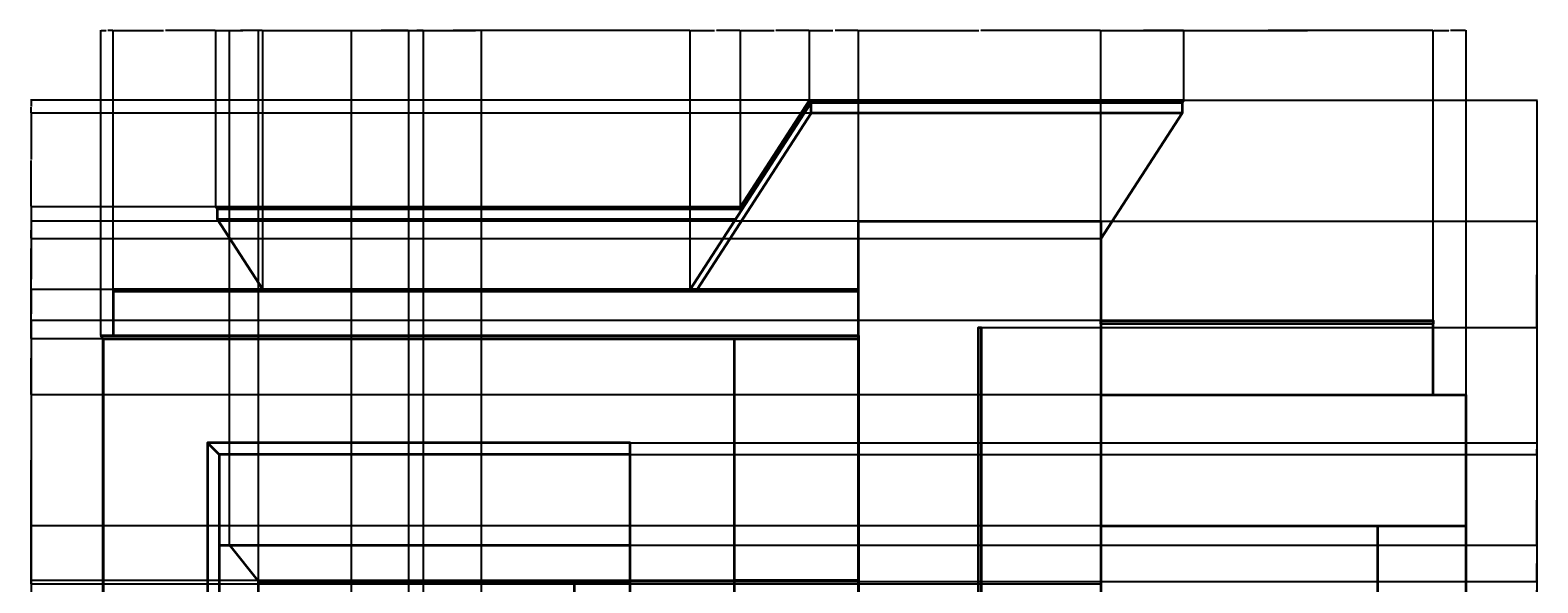
# Model space of a CAD drawing. Units: feet. Extents: x 4092 to 5585, y 725 to 1390.
# Tile 7 of 7: x 4921 to 5585, y 1146 to 1390. Entities that reach past the tile are written whole.
import ezdxf

# ---------------------------------------------------------------- set-up
doc = ezdxf.new("R2010")
doc.units = ezdxf.units.FT
doc.layers.add('A-ANNO-DIMS', color=2, linetype='Continuous', lineweight=18)
doc.layers.add('A-ELEV', color=7, linetype='Continuous', lineweight=35)
doc.styles.get("Standard").update_dxf_attribs({"font": 'arial.ttf'})
doc.dimstyles.get("Standard").update_dxf_attribs({"dimtxt": 0.18, "dimasz": 0.18, "dimexe": 0.18, "dimexo": 0.0625, "dimgap": 0.09, "dimtad": 0, "dimtih": 1, "dimtoh": 1, "dimdec": 1, "dimzin": 0, "dimdsep": 46, "dimlunit": 3, "dimtxsty": 'Standard', "dimcen": 0.09, "dimadec": 0, "dimazin": 0, "dimtfac": 1, "dimtdec": 1, "dimtofl": 0, "dimtmove": 0, "dimatfit": 3, "dimfxl": 1, "dimtolj": 1, "dimtzin": 0, "dimarcsym": 0})

# ---------------------------------------------------------------- blocks, each defined once
blk = doc.blocks.new('*D5')
at = {"layer": 'A-ANNO-DIMS', "color": 0, "lineweight": -2, "transparency": 16777216}
for p, q in [((5264.26, 1358.97), (5584.71, 1358.97)), ((5584.53, 1358.79), (5584.53, 1057.64)), ((5584.53, 756.13), (5584.53, 1057.28)), ((5553.36, 755.95), (5584.71, 755.95))]:
    blk.add_line(p, q, dxfattribs=at)
at = {"layer": 'A-ANNO-DIMS', "color": 0, "transparency": 16777216}
for points in [[(5584.5, 1358.79), (5584.56, 1358.79), (5584.53, 1358.97)], [(5584.5, 756.13), (5584.56, 756.13), (5584.53, 755.95)]]:
    blk.add_solid(points, dxfattribs=at)
at = {"layer": 'Defpoints', "color": 0, "transparency": 16777216}
for p in [(5264.2, 1358.97), (5584.53, 1358.97), (5553.29, 755.95)]:
    blk.add_point(p, dxfattribs=at)
at = {"layer": 'A-ANNO-DIMS', "color": 0, "transparency": 16777216, "insert": (5584.53, 1057.46), "char_height": 0.18, "attachment_point": 5}
blk.add_mtext('\\A1;603', dxfattribs=at)
blk = doc.blocks.new('*D6')
at = {"layer": 'A-ANNO-DIMS', "color": 0, "lineweight": -2, "transparency": 16777216}
for p, q in [((4952.15, 1255.43), (4952.15, 1389.85)), ((4952.33, 1389.67), (4954.5, 1389.67)), ((4957.45, 1389.67), (4955.28, 1389.67)), ((4957.63, 1275.65), (4957.63, 1389.85))]:
    blk.add_line(p, q, dxfattribs=at)
at = {"layer": 'A-ANNO-DIMS', "color": 0, "transparency": 16777216}
for points in [[(4952.33, 1389.7), (4952.33, 1389.64), (4952.15, 1389.67)], [(4957.45, 1389.7), (4957.45, 1389.64), (4957.63, 1389.67)]]:
    blk.add_solid(points, dxfattribs=at)
at = {"layer": 'Defpoints', "color": 0, "transparency": 16777216}
for p in [(4957.63, 1389.67), (4957.63, 1275.59), (4952.15, 1255.37)]:
    blk.add_point(p, dxfattribs=at)
at = {"layer": 'A-ANNO-DIMS', "color": 0, "transparency": 16777216, "insert": (4954.89, 1389.67), "char_height": 0.18, "attachment_point": 5}
blk.add_mtext('\\A1;5.475', dxfattribs=at)
blk = doc.blocks.new('*D7')
at = {"layer": 'A-ANNO-DIMS', "color": 0, "lineweight": -2, "transparency": 16777216}
for p, q in [((4957.63, 1275.65), (4957.63, 1389.85)), ((4957.81, 1389.67), (4979.82, 1389.67)), ((5002.64, 1389.67), (4980.62, 1389.67)), ((5002.82, 1312.19), (5002.82, 1389.85))]:
    blk.add_line(p, q, dxfattribs=at)
at = {"layer": 'A-ANNO-DIMS', "color": 0, "transparency": 16777216}
for points in [[(4957.81, 1389.7), (4957.81, 1389.64), (4957.63, 1389.67)], [(5002.64, 1389.7), (5002.64, 1389.64), (5002.82, 1389.67)]]:
    blk.add_solid(points, dxfattribs=at)
at = {"layer": 'Defpoints', "color": 0, "transparency": 16777216}
for p in [(5002.82, 1389.67), (5002.82, 1312.12), (4957.63, 1275.59)]:
    blk.add_point(p, dxfattribs=at)
at = {"layer": 'A-ANNO-DIMS', "color": 0, "transparency": 16777216, "insert": (4980.22, 1389.67), "char_height": 0.18, "attachment_point": 5}
blk.add_mtext('\\A1;45.19', dxfattribs=at)
blk = doc.blocks.new('*D8')
at = {"layer": 'A-ANNO-DIMS', "color": 0, "lineweight": -2, "transparency": 16777216}
for p, q in [((5002.82, 1312.19), (5002.82, 1389.85)), ((5003, 1389.67), (5012.71, 1389.67)), ((5023.35, 1389.67), (5013.64, 1389.67)), ((5023.53, 1275.65), (5023.53, 1389.85))]:
    blk.add_line(p, q, dxfattribs=at)
at = {"layer": 'A-ANNO-DIMS', "color": 0, "transparency": 16777216}
for points in [[(5003, 1389.7), (5003, 1389.64), (5002.82, 1389.67)], [(5023.35, 1389.7), (5023.35, 1389.64), (5023.53, 1389.67)]]:
    blk.add_solid(points, dxfattribs=at)
at = {"layer": 'Defpoints', "color": 0, "transparency": 16777216}
for p in [(5023.53, 1389.67), (5002.82, 1312.12), (5023.53, 1275.59)]:
    blk.add_point(p, dxfattribs=at)
at = {"layer": 'A-ANNO-DIMS', "color": 0, "transparency": 16777216, "insert": (5013.17, 1389.67), "char_height": 0.18, "attachment_point": 5}
blk.add_mtext('\\A1;20.714', dxfattribs=at)
blk = doc.blocks.new('*D9')
at = {"layer": 'A-ANNO-DIMS', "color": 0, "lineweight": -2, "transparency": 16777216}
for p, q in [((5023.53, 1275.65), (5023.53, 1389.85)), ((5023.71, 1389.67), (5117.14, 1389.67)), ((5211.48, 1389.67), (5118.05, 1389.67)), ((5211.66, 1275.65), (5211.66, 1389.85))]:
    blk.add_line(p, q, dxfattribs=at)
at = {"layer": 'A-ANNO-DIMS', "color": 0, "transparency": 16777216}
for points in [[(5023.71, 1389.7), (5023.71, 1389.64), (5023.53, 1389.67)], [(5211.48, 1389.7), (5211.48, 1389.64), (5211.66, 1389.67)]]:
    blk.add_solid(points, dxfattribs=at)
at = {"layer": 'Defpoints', "color": 0, "transparency": 16777216}
for p in [(5211.66, 1389.67), (5023.53, 1275.59), (5211.66, 1275.59)]:
    blk.add_point(p, dxfattribs=at)
at = {"layer": 'A-ANNO-DIMS', "color": 0, "transparency": 16777216, "insert": (5117.6, 1389.67), "char_height": 0.18, "attachment_point": 5}
blk.add_mtext('\\A1;188.13', dxfattribs=at)
blk = doc.blocks.new('*D10')
at = {"layer": 'A-ANNO-DIMS', "color": 0, "lineweight": -2, "transparency": 16777216}
for p, q in [((5211.66, 1275.65), (5211.66, 1389.85)), ((5211.84, 1389.67), (5222.32, 1389.67)), ((5233.73, 1389.67), (5223.25, 1389.67)), ((5233.91, 1312.19), (5233.91, 1389.85))]:
    blk.add_line(p, q, dxfattribs=at)
at = {"layer": 'A-ANNO-DIMS', "color": 0, "transparency": 16777216}
for points in [[(5211.84, 1389.7), (5211.84, 1389.64), (5211.66, 1389.67)], [(5233.73, 1389.7), (5233.73, 1389.64), (5233.91, 1389.67)]]:
    blk.add_solid(points, dxfattribs=at)
at = {"layer": 'Defpoints', "color": 0, "transparency": 16777216}
for p in [(5233.91, 1389.67), (5233.91, 1312.12), (5211.66, 1275.59)]:
    blk.add_point(p, dxfattribs=at)
at = {"layer": 'A-ANNO-DIMS', "color": 0, "transparency": 16777216, "insert": (5222.78, 1389.67), "char_height": 0.18, "attachment_point": 5}
blk.add_mtext('\\A1;22.248', dxfattribs=at)
blk = doc.blocks.new('*D11')
at = {"layer": 'A-ANNO-DIMS', "color": 0, "lineweight": -2, "transparency": 16777216}
for p, q in [((5233.91, 1312.19), (5233.91, 1389.85)), ((5234.09, 1389.67), (5248.66, 1389.67)), ((5264.02, 1389.67), (5249.45, 1389.67)), ((5264.2, 1359.04), (5264.2, 1389.85))]:
    blk.add_line(p, q, dxfattribs=at)
at = {"layer": 'A-ANNO-DIMS', "color": 0, "transparency": 16777216}
for points in [[(5234.09, 1389.7), (5234.09, 1389.64), (5233.91, 1389.67)], [(5264.02, 1389.7), (5264.02, 1389.64), (5264.2, 1389.67)]]:
    blk.add_solid(points, dxfattribs=at)
at = {"layer": 'Defpoints', "color": 0, "transparency": 16777216}
for p in [(5264.2, 1389.67), (5264.2, 1358.97), (5233.91, 1312.12)]:
    blk.add_point(p, dxfattribs=at)
at = {"layer": 'A-ANNO-DIMS', "color": 0, "transparency": 16777216, "insert": (5249.05, 1389.67), "char_height": 0.18, "attachment_point": 5}
blk.add_mtext('\\A1;30.29', dxfattribs=at)
blk = doc.blocks.new('*D12')
at = {"layer": 'A-ANNO-DIMS', "color": 0, "lineweight": -2, "transparency": 16777216}
for p, q in [((5264.2, 1359.04), (5264.2, 1389.85)), ((5264.38, 1389.67), (5274.53, 1389.67)), ((5285.61, 1389.67), (5275.46, 1389.67)), ((5285.79, 1305.84), (5285.79, 1389.85))]:
    blk.add_line(p, q, dxfattribs=at)
at = {"layer": 'A-ANNO-DIMS', "color": 0, "transparency": 16777216}
for points in [[(5264.38, 1389.7), (5264.38, 1389.64), (5264.2, 1389.67)], [(5285.61, 1389.7), (5285.61, 1389.64), (5285.79, 1389.67)]]:
    blk.add_solid(points, dxfattribs=at)
at = {"layer": 'Defpoints', "color": 0, "transparency": 16777216}
for p in [(5285.79, 1389.67), (5264.2, 1358.97), (5285.79, 1305.77)]:
    blk.add_point(p, dxfattribs=at)
at = {"layer": 'A-ANNO-DIMS', "color": 0, "transparency": 16777216, "insert": (5274.99, 1389.67), "char_height": 0.18, "attachment_point": 5}
blk.add_mtext('\\A1;21.594', dxfattribs=at)
blk = doc.blocks.new('*D13')
at = {"layer": 'A-ANNO-DIMS', "color": 0, "lineweight": -2, "transparency": 16777216}
for p, q in [((5285.79, 1305.84), (5285.79, 1389.85)), ((5285.97, 1389.67), (5338.72, 1389.67)), ((5392.37, 1389.67), (5339.63, 1389.67)), ((5392.55, 1305.84), (5392.55, 1389.85))]:
    blk.add_line(p, q, dxfattribs=at)
at = {"layer": 'A-ANNO-DIMS', "color": 0, "transparency": 16777216}
for points in [[(5285.97, 1389.7), (5285.97, 1389.64), (5285.79, 1389.67)], [(5392.37, 1389.7), (5392.37, 1389.64), (5392.55, 1389.67)]]:
    blk.add_solid(points, dxfattribs=at)
at = {"layer": 'Defpoints', "color": 0, "transparency": 16777216}
for p in [(5392.55, 1389.67), (5285.79, 1305.77), (5392.55, 1305.77)]:
    blk.add_point(p, dxfattribs=at)
at = {"layer": 'A-ANNO-DIMS', "color": 0, "transparency": 16777216, "insert": (5339.17, 1389.67), "char_height": 0.18, "attachment_point": 5}
blk.add_mtext('\\A1;106.76', dxfattribs=at)
blk = doc.blocks.new('*D14')
at = {"layer": 'A-ANNO-DIMS', "color": 0, "lineweight": -2, "transparency": 16777216}
for p, q in [((5392.55, 1305.84), (5392.55, 1389.85)), ((5392.73, 1389.67), (5410.44, 1389.67)), ((5428.93, 1389.67), (5411.23, 1389.67)), ((5429.11, 1359.04), (5429.11, 1389.85))]:
    blk.add_line(p, q, dxfattribs=at)
at = {"layer": 'A-ANNO-DIMS', "color": 0, "transparency": 16777216}
for points in [[(5392.73, 1389.7), (5392.73, 1389.64), (5392.55, 1389.67)], [(5428.93, 1389.7), (5428.93, 1389.64), (5429.11, 1389.67)]]:
    blk.add_solid(points, dxfattribs=at)
at = {"layer": 'Defpoints', "color": 0, "transparency": 16777216}
for p in [(5429.11, 1389.67), (5429.11, 1358.97), (5392.55, 1305.77)]:
    blk.add_point(p, dxfattribs=at)
at = {"layer": 'A-ANNO-DIMS', "color": 0, "transparency": 16777216, "insert": (5410.83, 1389.67), "char_height": 0.18, "attachment_point": 5}
blk.add_mtext('\\A1;36.56', dxfattribs=at)
blk = doc.blocks.new('*D15')
at = {"layer": 'A-ANNO-DIMS', "color": 0, "lineweight": -2, "transparency": 16777216}
for p, q in [((5429.11, 1359.04), (5429.11, 1389.85)), ((5429.29, 1389.67), (5483.54, 1389.67)), ((5538.7, 1389.67), (5484.45, 1389.67)), ((5538.88, 1262.03), (5538.88, 1389.85))]:
    blk.add_line(p, q, dxfattribs=at)
at = {"layer": 'A-ANNO-DIMS', "color": 0, "transparency": 16777216}
for points in [[(5429.29, 1389.7), (5429.29, 1389.64), (5429.11, 1389.67)], [(5538.7, 1389.7), (5538.7, 1389.64), (5538.88, 1389.67)]]:
    blk.add_solid(points, dxfattribs=at)
at = {"layer": 'Defpoints', "color": 0, "transparency": 16777216}
for p in [(5538.88, 1389.67), (5429.11, 1358.97), (5538.88, 1261.97)]:
    blk.add_point(p, dxfattribs=at)
at = {"layer": 'A-ANNO-DIMS', "color": 0, "transparency": 16777216, "insert": (5484, 1389.67), "char_height": 0.18, "attachment_point": 5}
blk.add_mtext('\\A1;109.77', dxfattribs=at)
blk = doc.blocks.new('*D16')
at = {"layer": 'A-ANNO-DIMS', "color": 0, "lineweight": -2, "transparency": 16777216}
for p, q in [((5538.88, 1262.03), (5538.88, 1389.85)), ((5539.06, 1389.67), (5545.72, 1389.67)), ((5553.11, 1389.67), (5546.46, 1389.67)), ((5553.29, 1229.33), (5553.29, 1389.85))]:
    blk.add_line(p, q, dxfattribs=at)
at = {"layer": 'A-ANNO-DIMS', "color": 0, "transparency": 16777216}
for points in [[(5539.06, 1389.7), (5539.06, 1389.64), (5538.88, 1389.67)], [(5553.11, 1389.7), (5553.11, 1389.64), (5553.29, 1389.67)]]:
    blk.add_solid(points, dxfattribs=at)
at = {"layer": 'Defpoints', "color": 0, "transparency": 16777216}
for p in [(5553.29, 1389.67), (5538.88, 1261.97), (5553.29, 1229.27)]:
    blk.add_point(p, dxfattribs=at)
at = {"layer": 'A-ANNO-DIMS', "color": 0, "transparency": 16777216, "insert": (5546.09, 1389.67), "char_height": 0.18, "attachment_point": 5}
blk.add_mtext('\\A1;14.41', dxfattribs=at)
blk = doc.blocks.new('*D19')
at = {"layer": 'A-ANNO-DIMS', "color": 0, "lineweight": -2, "transparency": 16777216}
for p, q in [((4953.23, 1253.95), (4921.27, 1253.95)), ((4921.45, 1253.77), (4921.45, 1132.55)), ((4921.45, 1010.97), (4921.45, 1132.19)), ((4978.29, 1010.79), (4921.27, 1010.79))]:
    blk.add_line(p, q, dxfattribs=at)
at = {"layer": 'A-ANNO-DIMS', "color": 0, "transparency": 16777216}
for points in [[(4921.42, 1253.77), (4921.48, 1253.77), (4921.45, 1253.95)], [(4921.42, 1010.97), (4921.48, 1010.97), (4921.45, 1010.79)]]:
    blk.add_solid(points, dxfattribs=at)
at = {"layer": 'Defpoints', "color": 0, "transparency": 16777216}
for p in [(4921.45, 1253.95), (4953.29, 1253.95), (4978.36, 1010.79)]:
    blk.add_point(p, dxfattribs=at)
at = {"layer": 'A-ANNO-DIMS', "color": 0, "transparency": 16777216, "insert": (4921.45, 1132.37), "char_height": 0.18, "attachment_point": 5}
blk.add_mtext('\\A1;243.16', dxfattribs=at)
blk = doc.blocks.new('*D20')
at = {"layer": 'A-ANNO-DIMS', "color": 0, "lineweight": -2, "transparency": 16777216}
for p, q in [((4957.56, 1275.59), (4921.27, 1275.59)), ((4921.45, 1275.41), (4921.45, 1264.95)), ((4921.45, 1254.13), (4921.45, 1264.59)), ((4953.23, 1253.95), (4921.27, 1253.95))]:
    blk.add_line(p, q, dxfattribs=at)
at = {"layer": 'A-ANNO-DIMS', "color": 0, "transparency": 16777216}
for points in [[(4921.42, 1275.41), (4921.48, 1275.41), (4921.45, 1275.59)], [(4921.42, 1254.13), (4921.48, 1254.13), (4921.45, 1253.95)]]:
    blk.add_solid(points, dxfattribs=at)
at = {"layer": 'Defpoints', "color": 0, "transparency": 16777216}
for p in [(4921.45, 1275.59), (4957.63, 1275.59), (4953.29, 1253.95)]:
    blk.add_point(p, dxfattribs=at)
at = {"layer": 'A-ANNO-DIMS', "color": 0, "transparency": 16777216, "insert": (4921.45, 1264.77), "char_height": 0.18, "attachment_point": 5}
blk.add_mtext('\\A1;21.64', dxfattribs=at)
blk = doc.blocks.new('*D21')
at = {"layer": 'A-ANNO-DIMS', "color": 0, "lineweight": -2, "transparency": 16777216}
for p, q in [((5002.75, 1312.12), (4921.27, 1312.12)), ((4921.45, 1311.94), (4921.45, 1294.04)), ((4921.45, 1275.77), (4921.45, 1293.67)), ((4957.56, 1275.59), (4921.27, 1275.59))]:
    blk.add_line(p, q, dxfattribs=at)
at = {"layer": 'A-ANNO-DIMS', "color": 0, "transparency": 16777216}
for points in [[(4921.42, 1311.94), (4921.48, 1311.94), (4921.45, 1312.12)], [(4921.42, 1275.77), (4921.48, 1275.77), (4921.45, 1275.59)]]:
    blk.add_solid(points, dxfattribs=at)
at = {"layer": 'Defpoints', "color": 0, "transparency": 16777216}
for p in [(4921.45, 1312.12), (5002.82, 1312.12), (4957.63, 1275.59)]:
    blk.add_point(p, dxfattribs=at)
at = {"layer": 'A-ANNO-DIMS', "color": 0, "transparency": 16777216, "insert": (4921.45, 1293.86), "char_height": 0.18, "attachment_point": 5}
blk.add_mtext('\\A1;36.534', dxfattribs=at)
blk = doc.blocks.new('*D22')
at = {"layer": 'A-ANNO-DIMS', "color": 0, "lineweight": -2, "transparency": 16777216}
for p, q in [((5264.87, 1353.23), (4921.27, 1353.23)), ((4921.45, 1353.05), (4921.45, 1332.85)), ((4921.45, 1312.3), (4921.45, 1332.49)), ((5002.75, 1312.12), (4921.27, 1312.12))]:
    blk.add_line(p, q, dxfattribs=at)
at = {"layer": 'A-ANNO-DIMS', "color": 0, "transparency": 16777216}
for points in [[(4921.42, 1353.05), (4921.48, 1353.05), (4921.45, 1353.23)], [(4921.42, 1312.3), (4921.48, 1312.3), (4921.45, 1312.12)]]:
    blk.add_solid(points, dxfattribs=at)
at = {"layer": 'Defpoints', "color": 0, "transparency": 16777216}
for p in [(4921.45, 1353.23), (5264.93, 1353.23), (5002.82, 1312.12)]:
    blk.add_point(p, dxfattribs=at)
at = {"layer": 'A-ANNO-DIMS', "color": 0, "transparency": 16777216, "insert": (4921.45, 1332.67), "char_height": 0.18, "attachment_point": 5}
blk.add_mtext('\\A1;41.1', dxfattribs=at)
blk = doc.blocks.new('*D23')
at = {"layer": 'A-ANNO-DIMS', "color": 0, "lineweight": -2, "transparency": 16777216}
for p, q in [((5264.14, 1358.97), (4921.27, 1358.97)), ((4921.45, 1358.79), (4921.45, 1356.28)), ((4921.45, 1353.41), (4921.45, 1355.92)), ((5264.87, 1353.23), (4921.27, 1353.23))]:
    blk.add_line(p, q, dxfattribs=at)
at = {"layer": 'A-ANNO-DIMS', "color": 0, "transparency": 16777216}
for points in [[(4921.42, 1358.79), (4921.48, 1358.79), (4921.45, 1358.97)], [(4921.42, 1353.41), (4921.48, 1353.41), (4921.45, 1353.23)]]:
    blk.add_solid(points, dxfattribs=at)
at = {"layer": 'Defpoints', "color": 0, "transparency": 16777216}
for p in [(4921.45, 1358.97), (5264.2, 1358.97), (5264.93, 1353.23)]:
    blk.add_point(p, dxfattribs=at)
at = {"layer": 'A-ANNO-DIMS', "color": 0, "transparency": 16777216, "insert": (4921.45, 1356.1), "char_height": 0.18, "attachment_point": 5}
blk.add_mtext('\\A1;5.747', dxfattribs=at)
blk = doc.blocks.new('*D39')
at = {"layer": 'A-ANNO-DIMS', "color": 0, "lineweight": -2, "transparency": 16777216}
for p, q in [((5087.84, 808.72), (5087.84, 1389.85)), ((5088.02, 1389.67), (5090.69, 1389.67)), ((5094.12, 1389.67), (5091.45, 1389.67)), ((5094.3, 808.72), (5094.3, 1389.85))]:
    blk.add_line(p, q, dxfattribs=at)
at = {"layer": 'A-ANNO-DIMS', "color": 0, "transparency": 16777216}
for points in [[(5088.02, 1389.7), (5088.02, 1389.64), (5087.84, 1389.67)], [(5094.12, 1389.7), (5094.12, 1389.64), (5094.3, 1389.67)]]:
    blk.add_solid(points, dxfattribs=at)
at = {"layer": 'Defpoints', "color": 0, "transparency": 16777216}
for p in [(5094.3, 1389.67), (5087.84, 808.65), (5094.3, 808.65)]:
    blk.add_point(p, dxfattribs=at)
at = {"layer": 'A-ANNO-DIMS', "color": 0, "transparency": 16777216, "insert": (5091.07, 1389.67), "char_height": 0.18, "attachment_point": 5}
blk.add_mtext('\\A1;6.461', dxfattribs=at)
blk = doc.blocks.new('*D40')
at = {"layer": 'A-ANNO-DIMS', "color": 0, "lineweight": -2, "transparency": 16777216}
for p, q in [((5062.58, 907.22), (5062.58, 1389.85)), ((5062.76, 1389.67), (5074.7, 1389.67)), ((5087.57, 1389.67), (5075.63, 1389.67)), ((5087.75, 907.22), (5087.75, 1389.85))]:
    blk.add_line(p, q, dxfattribs=at)
at = {"layer": 'A-ANNO-DIMS', "color": 0, "transparency": 16777216}
for points in [[(5062.76, 1389.7), (5062.76, 1389.64), (5062.58, 1389.67)], [(5087.57, 1389.7), (5087.57, 1389.64), (5087.75, 1389.67)]]:
    blk.add_solid(points, dxfattribs=at)
at = {"layer": 'Defpoints', "color": 0, "transparency": 16777216}
for p in [(5087.75, 1389.67), (5062.58, 907.16), (5087.75, 907.16)]:
    blk.add_point(p, dxfattribs=at)
at = {"layer": 'A-ANNO-DIMS', "color": 0, "transparency": 16777216, "insert": (5075.16, 1389.67), "char_height": 0.18, "attachment_point": 5}
blk.add_mtext('\\A1;25.164', dxfattribs=at)
blk = doc.blocks.new('*D41')
at = {"layer": 'A-ANNO-DIMS', "color": 0, "lineweight": -2, "transparency": 16777216}
for p, q in [((5087.75, 907.22), (5087.75, 1389.85)), ((5087.93, 1389.67), (5090.59, 1389.67)), ((5094.04, 1389.67), (5091.38, 1389.67)), ((5094.22, 907.22), (5094.22, 1389.85))]:
    blk.add_line(p, q, dxfattribs=at)
at = {"layer": 'A-ANNO-DIMS', "color": 0, "transparency": 16777216}
for points in [[(5087.93, 1389.7), (5087.93, 1389.64), (5087.75, 1389.67)], [(5094.04, 1389.7), (5094.04, 1389.64), (5094.22, 1389.67)]]:
    blk.add_solid(points, dxfattribs=at)
at = {"layer": 'Defpoints', "color": 0, "transparency": 16777216}
for p in [(5094.22, 1389.67), (5087.75, 907.16), (5094.22, 907.16)]:
    blk.add_point(p, dxfattribs=at)
at = {"layer": 'A-ANNO-DIMS', "color": 0, "transparency": 16777216, "insert": (5090.98, 1389.67), "char_height": 0.18, "attachment_point": 5}
blk.add_mtext('\\A1;6.474', dxfattribs=at)
blk = doc.blocks.new('*D42')
at = {"layer": 'A-ANNO-DIMS', "color": 0, "lineweight": -2, "transparency": 16777216}
for p, q in [((5094.22, 907.22), (5094.22, 1389.85)), ((5094.4, 1389.67), (5106.69, 1389.67)), ((5119.64, 1389.67), (5107.34, 1389.67)), ((5119.82, 907.22), (5119.82, 1389.85))]:
    blk.add_line(p, q, dxfattribs=at)
at = {"layer": 'A-ANNO-DIMS', "color": 0, "transparency": 16777216}
for points in [[(5094.4, 1389.7), (5094.4, 1389.64), (5094.22, 1389.67)], [(5119.64, 1389.7), (5119.64, 1389.64), (5119.82, 1389.67)]]:
    blk.add_solid(points, dxfattribs=at)
at = {"layer": 'Defpoints', "color": 0, "transparency": 16777216}
for p in [(5119.82, 1389.67), (5094.22, 907.16), (5119.82, 907.16)]:
    blk.add_point(p, dxfattribs=at)
at = {"layer": 'A-ANNO-DIMS', "color": 0, "transparency": 16777216, "insert": (5107.02, 1389.67), "char_height": 0.18, "attachment_point": 5}
blk.add_mtext('\\A1;25.6', dxfattribs=at)
blk = doc.blocks.new('*D59')
at = {"layer": 'A-ANNO-DIMS', "color": 0, "lineweight": -2, "transparency": 16777216}
for p, q in [((5185.39, 1147.07), (5584.71, 1147.07)), ((5584.53, 1146.89), (5584.53, 1143.66)), ((5584.53, 1140.06), (5584.53, 1143.3)), ((5153.4, 1139.88), (5584.71, 1139.88))]:
    blk.add_line(p, q, dxfattribs=at)
at = {"layer": 'A-ANNO-DIMS', "color": 0, "transparency": 16777216}
for points in [[(5584.5, 1146.89), (5584.56, 1146.89), (5584.53, 1147.07)], [(5584.5, 1140.06), (5584.56, 1140.06), (5584.53, 1139.88)]]:
    blk.add_solid(points, dxfattribs=at)
at = {"layer": 'Defpoints', "color": 0, "transparency": 16777216}
for p in [(5185.33, 1147.07), (5584.53, 1147.07), (5153.34, 1139.88)]:
    blk.add_point(p, dxfattribs=at)
at = {"layer": 'A-ANNO-DIMS', "color": 0, "transparency": 16777216, "insert": (5584.53, 1143.48), "char_height": 0.18, "attachment_point": 5}
blk.add_mtext('\\A1;7.194', dxfattribs=at)
blk = doc.blocks.new('*D60')
at = {"layer": 'A-ANNO-DIMS', "color": 0, "lineweight": -2, "transparency": 16777216}
for p, q in [((5185.39, 1163.13), (5584.71, 1163.13)), ((5584.53, 1162.95), (5584.53, 1155.28)), ((5584.53, 1147.25), (5584.53, 1154.92)), ((5185.39, 1147.07), (5584.71, 1147.07))]:
    blk.add_line(p, q, dxfattribs=at)
at = {"layer": 'A-ANNO-DIMS', "color": 0, "transparency": 16777216}
for points in [[(5584.5, 1162.95), (5584.56, 1162.95), (5584.53, 1163.13)], [(5584.5, 1147.25), (5584.56, 1147.25), (5584.53, 1147.07)]]:
    blk.add_solid(points, dxfattribs=at)
at = {"layer": 'Defpoints', "color": 0, "transparency": 16777216}
for p in [(5185.33, 1163.13), (5584.53, 1163.13), (5185.33, 1147.07)]:
    blk.add_point(p, dxfattribs=at)
at = {"layer": 'A-ANNO-DIMS', "color": 0, "transparency": 16777216, "insert": (5584.53, 1155.1), "char_height": 0.18, "attachment_point": 5}
blk.add_mtext('\\A1;16.057', dxfattribs=at)
blk = doc.blocks.new('*D61')
at = {"layer": 'A-ANNO-DIMS', "color": 0, "lineweight": -2, "transparency": 16777216}
for p, q in [((5185.39, 1202.92), (5584.71, 1202.92)), ((5584.53, 1202.74), (5584.53, 1183.21)), ((5584.53, 1163.31), (5584.53, 1182.85)), ((5185.39, 1163.13), (5584.71, 1163.13))]:
    blk.add_line(p, q, dxfattribs=at)
at = {"layer": 'A-ANNO-DIMS', "color": 0, "transparency": 16777216}
for points in [[(5584.5, 1202.74), (5584.56, 1202.74), (5584.53, 1202.92)], [(5584.5, 1163.31), (5584.56, 1163.31), (5584.53, 1163.13)]]:
    blk.add_solid(points, dxfattribs=at)
at = {"layer": 'Defpoints', "color": 0, "transparency": 16777216}
for p in [(5185.33, 1202.92), (5584.53, 1202.92), (5185.33, 1163.13)]:
    blk.add_point(p, dxfattribs=at)
at = {"layer": 'A-ANNO-DIMS', "color": 0, "transparency": 16777216, "insert": (5584.53, 1183.03), "char_height": 0.18, "attachment_point": 5}
blk.add_mtext('\\A1;39.79', dxfattribs=at)
blk = doc.blocks.new('*D62')
at = {"layer": 'A-ANNO-DIMS', "color": 0, "lineweight": -2, "transparency": 16777216}
for p, q in [((5185.39, 1208.13), (5584.71, 1208.13)), ((5185.39, 1202.92), (5584.71, 1202.92)), ((5584.53, 1207.95), (5584.53, 1205.71)), ((5584.53, 1203.1), (5584.53, 1205.34))]:
    blk.add_line(p, q, dxfattribs=at)
at = {"layer": 'A-ANNO-DIMS', "color": 0, "transparency": 16777216}
for points in [[(5584.5, 1207.95), (5584.56, 1207.95), (5584.53, 1208.13)], [(5584.5, 1203.1), (5584.56, 1203.1), (5584.53, 1202.92)]]:
    blk.add_solid(points, dxfattribs=at)
at = {"layer": 'Defpoints', "color": 0, "transparency": 16777216}
for p in [(5185.33, 1208.13), (5185.33, 1202.92), (5584.53, 1208.13)]:
    blk.add_point(p, dxfattribs=at)
at = {"layer": 'A-ANNO-DIMS', "color": 0, "transparency": 16777216, "insert": (5584.53, 1205.53), "char_height": 0.18, "attachment_point": 5}
blk.add_mtext('\\A1;5.203', dxfattribs=at)
blk = doc.blocks.new('*D63')
at = {"layer": 'A-ANNO-DIMS', "color": 0, "lineweight": -2, "transparency": 16777216}
for p, q in [((5008.84, 1163.19), (5008.84, 1389.85)), ((5009.02, 1389.67), (5014.77, 1389.67)), ((5021.43, 1389.67), (5015.68, 1389.67)), ((5021.61, 1147.14), (5021.61, 1389.85))]:
    blk.add_line(p, q, dxfattribs=at)
at = {"layer": 'A-ANNO-DIMS', "color": 0, "transparency": 16777216}
for points in [[(5009.02, 1389.7), (5009.02, 1389.64), (5008.84, 1389.67)], [(5021.43, 1389.7), (5021.43, 1389.64), (5021.61, 1389.67)]]:
    blk.add_solid(points, dxfattribs=at)
at = {"layer": 'Defpoints', "color": 0, "transparency": 16777216}
for p in [(5021.61, 1389.67), (5008.84, 1163.13), (5021.61, 1147.07)]:
    blk.add_point(p, dxfattribs=at)
at = {"layer": 'A-ANNO-DIMS', "color": 0, "transparency": 16777216, "insert": (5015.22, 1389.67), "char_height": 0.18, "attachment_point": 5}
blk.add_mtext('\\A1;12.765', dxfattribs=at)
blk = doc.blocks.new('*D81')
at = {"layer": 'A-ANNO-DIMS', "color": 0, "lineweight": -2, "transparency": 16777216}
for p, q in [((5392.49, 1171.51), (4921.27, 1171.51)), ((4921.45, 1171.33), (4921.45, 1158.87)), ((4921.45, 1146.04), (4921.45, 1158.5)), ((5392.49, 1145.86), (4921.27, 1145.86))]:
    blk.add_line(p, q, dxfattribs=at)
at = {"layer": 'A-ANNO-DIMS', "color": 0, "transparency": 16777216}
for points in [[(4921.42, 1171.33), (4921.48, 1171.33), (4921.45, 1171.51)], [(4921.42, 1146.04), (4921.48, 1146.04), (4921.45, 1145.86)]]:
    blk.add_solid(points, dxfattribs=at)
at = {"layer": 'Defpoints', "color": 0, "transparency": 16777216}
for p in [(4921.45, 1171.51), (5392.55, 1171.51), (5392.55, 1145.86)]:
    blk.add_point(p, dxfattribs=at)
at = {"layer": 'A-ANNO-DIMS', "color": 0, "transparency": 16777216, "insert": (4921.45, 1158.69), "char_height": 0.18, "attachment_point": 5}
blk.add_mtext('\\A1;25.65', dxfattribs=at)
blk = doc.blocks.new('*D82')
at = {"layer": 'A-ANNO-DIMS', "color": 0, "lineweight": -2, "transparency": 16777216}
for p, q in [((5392.49, 1229.27), (4921.27, 1229.27)), ((4921.45, 1229.09), (4921.45, 1200.57)), ((4921.45, 1171.69), (4921.45, 1200.21)), ((5392.49, 1171.51), (4921.27, 1171.51))]:
    blk.add_line(p, q, dxfattribs=at)
at = {"layer": 'A-ANNO-DIMS', "color": 0, "transparency": 16777216}
for points in [[(4921.42, 1229.09), (4921.48, 1229.09), (4921.45, 1229.27)], [(4921.42, 1171.69), (4921.48, 1171.69), (4921.45, 1171.51)]]:
    blk.add_solid(points, dxfattribs=at)
at = {"layer": 'Defpoints', "color": 0, "transparency": 16777216}
for p in [(4921.45, 1229.27), (5392.55, 1229.27), (5392.55, 1171.51)]:
    blk.add_point(p, dxfattribs=at)
at = {"layer": 'A-ANNO-DIMS', "color": 0, "transparency": 16777216, "insert": (4921.45, 1200.39), "char_height": 0.18, "attachment_point": 5}
blk.add_mtext('\\A1;57.76', dxfattribs=at)
blk = doc.blocks.new('*D83')
at = {"layer": 'A-ANNO-DIMS', "color": 0, "lineweight": -2, "transparency": 16777216}
for p, q in [((5392.49, 1261.97), (4921.27, 1261.97)), ((4921.45, 1261.79), (4921.45, 1245.8)), ((4921.45, 1229.45), (4921.45, 1245.44)), ((5392.49, 1229.27), (4921.27, 1229.27))]:
    blk.add_line(p, q, dxfattribs=at)
at = {"layer": 'A-ANNO-DIMS', "color": 0, "transparency": 16777216}
for points in [[(4921.42, 1261.79), (4921.48, 1261.79), (4921.45, 1261.97)], [(4921.42, 1229.45), (4921.48, 1229.45), (4921.45, 1229.27)]]:
    blk.add_solid(points, dxfattribs=at)
at = {"layer": 'Defpoints', "color": 0, "transparency": 16777216}
for p in [(4921.45, 1261.97), (5392.55, 1261.97), (5392.55, 1229.27)]:
    blk.add_point(p, dxfattribs=at)
at = {"layer": 'A-ANNO-DIMS', "color": 0, "transparency": 16777216, "insert": (4921.45, 1245.62), "char_height": 0.18, "attachment_point": 5}
blk.add_mtext('\\A1;32.7', dxfattribs=at)
blk = doc.blocks.new('*D84')
at = {"layer": 'A-ANNO-DIMS', "color": 0, "lineweight": -2, "transparency": 16777216}
for p, q in [((5392.49, 1298.01), (4921.27, 1298.01)), ((4921.45, 1297.83), (4921.45, 1280.17)), ((4921.45, 1262.15), (4921.45, 1279.81)), ((5392.49, 1261.97), (4921.27, 1261.97))]:
    blk.add_line(p, q, dxfattribs=at)
at = {"layer": 'A-ANNO-DIMS', "color": 0, "transparency": 16777216}
for points in [[(4921.42, 1297.83), (4921.48, 1297.83), (4921.45, 1298.01)], [(4921.42, 1262.15), (4921.48, 1262.15), (4921.45, 1261.97)]]:
    blk.add_solid(points, dxfattribs=at)
at = {"layer": 'Defpoints', "color": 0, "transparency": 16777216}
for p in [(4921.45, 1298.01), (5392.55, 1298.01), (5392.55, 1261.97)]:
    blk.add_point(p, dxfattribs=at)
at = {"layer": 'A-ANNO-DIMS', "color": 0, "transparency": 16777216, "insert": (4921.45, 1279.99), "char_height": 0.18, "attachment_point": 5}
blk.add_mtext('\\A1;36.04', dxfattribs=at)
blk = doc.blocks.new('*D85')
at = {"layer": 'A-ANNO-DIMS', "color": 0, "lineweight": -2, "transparency": 16777216}
for p, q in [((5392.49, 1305.77), (4921.27, 1305.77)), ((4921.45, 1305.59), (4921.45, 1302.07)), ((4921.45, 1298.19), (4921.45, 1301.71)), ((5392.49, 1298.01), (4921.27, 1298.01))]:
    blk.add_line(p, q, dxfattribs=at)
at = {"layer": 'A-ANNO-DIMS', "color": 0, "transparency": 16777216}
for points in [[(4921.42, 1305.59), (4921.48, 1305.59), (4921.45, 1305.77)], [(4921.42, 1298.19), (4921.48, 1298.19), (4921.45, 1298.01)]]:
    blk.add_solid(points, dxfattribs=at)
at = {"layer": 'Defpoints', "color": 0, "transparency": 16777216}
for p in [(4921.45, 1305.77), (5392.55, 1305.77), (5392.55, 1298.01)]:
    blk.add_point(p, dxfattribs=at)
at = {"layer": 'A-ANNO-DIMS', "color": 0, "transparency": 16777216, "insert": (4921.45, 1301.89), "char_height": 0.18, "attachment_point": 5}
blk.add_mtext('\\A1;7.764', dxfattribs=at)
blk = doc.blocks.new('*D86')
at = {"layer": 'A-ANNO-DIMS', "color": 0, "lineweight": -2, "transparency": 16777216}
for p, q in [((5285.73, 1253.95), (4921.27, 1253.95)), ((4921.45, 1253.77), (4921.45, 1200.91)), ((4921.45, 1147.7), (4921.45, 1200.55)), ((5285.73, 1147.52), (4921.27, 1147.52))]:
    blk.add_line(p, q, dxfattribs=at)
at = {"layer": 'A-ANNO-DIMS', "color": 0, "transparency": 16777216}
for points in [[(4921.42, 1253.77), (4921.48, 1253.77), (4921.45, 1253.95)], [(4921.42, 1147.7), (4921.48, 1147.7), (4921.45, 1147.52)]]:
    blk.add_solid(points, dxfattribs=at)
at = {"layer": 'Defpoints', "color": 0, "transparency": 16777216}
for p in [(5285.79, 1253.95), (4921.45, 1147.52), (5285.79, 1147.52)]:
    blk.add_point(p, dxfattribs=at)
at = {"layer": 'A-ANNO-DIMS', "color": 0, "transparency": 16777216, "insert": (4921.45, 1200.73), "char_height": 0.18, "attachment_point": 5}
blk.add_mtext('\\A1;106.43', dxfattribs=at)
blk = doc.blocks.new('*D87')
at = {"layer": 'A-ANNO-DIMS', "color": 0, "lineweight": -2, "transparency": 16777216}
for p, q in [((5285.85, 1305.77), (5584.71, 1305.77)), ((5584.53, 1305.59), (5584.53, 1282.49)), ((5584.53, 1259.03), (5584.53, 1282.13)), ((5339.81, 1258.85), (5584.71, 1258.85))]:
    blk.add_line(p, q, dxfattribs=at)
at = {"layer": 'A-ANNO-DIMS', "color": 0, "transparency": 16777216}
for points in [[(5584.5, 1305.59), (5584.56, 1305.59), (5584.53, 1305.77)], [(5584.5, 1259.03), (5584.56, 1259.03), (5584.53, 1258.85)]]:
    blk.add_solid(points, dxfattribs=at)
at = {"layer": 'Defpoints', "color": 0, "transparency": 16777216}
for p in [(5285.79, 1305.77), (5339.75, 1258.85), (5584.53, 1258.85)]:
    blk.add_point(p, dxfattribs=at)
at = {"layer": 'A-ANNO-DIMS', "color": 0, "transparency": 16777216, "insert": (5584.53, 1282.31), "char_height": 0.18, "attachment_point": 5}
blk.add_mtext('\\A1;46.925', dxfattribs=at)
blk = doc.blocks.new('*D92')
at = {"layer": 'A-ANNO-DIMS', "color": 0, "lineweight": -2, "transparency": 16777216}
for p, q in [((5392.55, 1262.03), (5392.55, 1389.85)), ((5392.73, 1389.67), (5465.26, 1389.67)), ((5538.7, 1389.67), (5466.17, 1389.67)), ((5538.88, 1262.03), (5538.88, 1389.85))]:
    blk.add_line(p, q, dxfattribs=at)
at = {"layer": 'A-ANNO-DIMS', "color": 0, "transparency": 16777216}
for points in [[(5392.73, 1389.7), (5392.73, 1389.64), (5392.55, 1389.67)], [(5538.7, 1389.7), (5538.7, 1389.64), (5538.88, 1389.67)]]:
    blk.add_solid(points, dxfattribs=at)
at = {"layer": 'Defpoints', "color": 0, "transparency": 16777216}
for p in [(5538.88, 1389.67), (5392.55, 1261.97), (5538.88, 1261.97)]:
    blk.add_point(p, dxfattribs=at)
at = {"layer": 'A-ANNO-DIMS', "color": 0, "transparency": 16777216, "insert": (5465.72, 1389.67), "char_height": 0.18, "attachment_point": 5}
blk.add_mtext('\\A1;146.33', dxfattribs=at)

msp = doc.modelspace()

# ---------------------------------------------------------------- linework, layer by layer
at = {"layer": 'A-ELEV'}
for p, q in [((5264.9307, 1357.9844), (5211.6611, 1275.5883)), ((5264.1979, 1358.9731), (5233.9087, 1312.1225)), ((5264.9307, 1353.2259), (5264.9307, 1357.9844)), ((5428.2491, 1357.9844), (5429.1128, 1358.9731)), ((5264.9307, 1353.2259), (5214.7375, 1275.5883)), ((5428.2491, 1353.2259), (5392.5521, 1298.0107)), ((5003.5491, 1306.4942), (5023.53, 1275.5883)), ((4953.293, 1253.9488), (4952.1517, 1255.3673)), ((4953.293, 755.9488), (4953.293, 1253.9488)), ((4953.293, 1253.9488), (5285.7915, 1253.9488)), ((5392.5521, 1229.2703), (5553.293, 1229.2703)), ((5553.293, 755.9488), (5553.293, 1229.2703)), ((4999.1145, 1208.1273), (5004.3171, 1202.9247)), ((5392.5521, 1171.511), (5553.293, 1171.511)), ((5004.3171, 1163.131), (5185.3285, 1163.131)), ((5008.8415, 1163.131), (5021.6062, 1147.0743)), ((5160.5329, 1147.0743), (5185.3285, 1147.0743))]:
    msp.add_line(p, q, dxfattribs=at)
for points in [[(5428.2491, 1357.9844), (5264.9307, 1357.9844), (5264.1979, 1358.9731), (5429.1128, 1358.9731)], [(5264.9307, 1357.9844), (5428.2491, 1357.9844), (5428.2491, 1353.2259), (5264.9307, 1353.2259)], [(5234.6415, 1311.1338), (5003.5491, 1311.1338), (5002.8163, 1312.1225), (5235.2807, 1312.1225)], [(5231.6419, 1306.4942), (5003.5491, 1306.4942), (5003.5491, 1311.1338), (5234.6415, 1311.1338)], [(4952.1517, 1255.3673), (5285.7915, 1255.3673), (5285.7915, 1253.9488), (4953.293, 1253.9488)], [(5185.3285, 1010.7906), (5185.3285, 1208.1273), (4999.1145, 1208.1273), (4999.1145, 1010.7906)], [(5185.3285, 1202.9247), (5004.3171, 1202.9247), (5004.3171, 1010.7906)], [(5514.3304, 1171.511), (5514.3304, 1010.7906), (5392.5521, 1010.7906), (5392.5521, 1125.3426)], [(5021.6062, 1010.7906), (5021.6062, 1147.0743), (5160.5329, 1147.0743), (5160.5329, 1010.7906)]]:
    msp.add_lwpolyline(points, dxfattribs=at)
for points in [[(5392.5521, 755.9488), (5285.7915, 755.9488), (5285.7915, 1305.7746), (5392.5521, 1305.7746)], [(4957.6271, 1274.9372), (5285.7915, 1274.9372), (5285.7915, 1275.5883), (4957.6271, 1275.5883)], [(4957.6271, 1255.3673), (5285.7915, 1255.3673), (5285.7915, 1274.9372), (4957.6271, 1274.9372)], [(5538.8833, 1260.5931), (5392.5521, 1260.5931), (5392.5521, 1261.9705), (5538.8833, 1261.9705)], [(5338.5913, 820.9207), (5338.5913, 1258.8497), (5339.7523, 1258.8497), (5339.7523, 820.9207)], [(5392.5521, 1229.2703), (5538.8833, 1229.2703), (5538.8833, 1260.5931), (5392.5521, 1260.5931)], [(4953.293, 755.9488), (5231.15, 755.9488), (5231.15, 1253.9488), (4953.293, 1253.9488)], [(5231.15, 1253.9488), (5285.7915, 1253.9488), (5285.7915, 755.9488), (5231.15, 755.9488)], [(5231.15, 1253.9488), (5285.7915, 1253.9488), (5285.7915, 1147.5159), (5231.15, 1147.5159)]]:
    msp.add_lwpolyline(points, close=True, dxfattribs=at)

# ---------------------------------------------------------------- dimensions: what is measured, and where the dimension line sits
at = {"layer": 'A-ANNO-DIMS'}
for base, p1, p2, override, picture, middle in [((4957.6271, 1389.6731), (4952.1517, 1255.3673), (4957.6271, 1275.5883), {"dimdec": 3, "dimlfac": 1, "dimrnd": 0, "dimzin": 0, "dimdsep": 46, "dimlunit": 2}, '*D6', (4954.8894, 1389.6731)), ((5002.8163, 1389.6731), (4957.6271, 1275.5883), (5002.8163, 1312.1225), {"dimdec": 2, "dimlfac": 1, "dimrnd": 0, "dimzin": 0, "dimdsep": 46, "dimlunit": 2}, '*D7', (4980.2217, 1389.6731)), ((5023.53, 1389.6731), (5002.8163, 1312.1225), (5023.53, 1275.5883), {"dimdec": 3, "dimlfac": 1, "dimrnd": 0, "dimzin": 0, "dimdsep": 46, "dimlunit": 2}, '*D8', (5013.1731, 1389.6731)), ((5021.6062, 1389.6731), (5008.8415, 1163.131), (5021.6062, 1147.0743), {"dimdec": 3, "dimlfac": 1, "dimrnd": 0, "dimzin": 0, "dimdsep": 46, "dimlunit": 2}, '*D63', (5015.2238, 1389.6731)), ((5211.6611, 1389.6731), (5023.53, 1275.5883), (5211.6611, 1275.5883), {"dimdec": 2, "dimlfac": 1, "dimrnd": 0, "dimzin": 0, "dimdsep": 46, "dimlunit": 2}, '*D9', (5117.5955, 1389.6731)), ((5087.7457, 1389.6731), (5062.5819, 907.159), (5087.7457, 907.159), {"dimdec": 3, "dimlfac": 1, "dimrnd": 0, "dimzin": 0, "dimdsep": 46, "dimlunit": 2}, '*D40', (5075.1638, 1389.6731)), ((5094.2195, 1389.6731), (5087.7457, 907.159), (5094.2195, 907.159), {"dimdec": 3, "dimlfac": 1, "dimrnd": 0, "dimzin": 0, "dimdsep": 46, "dimlunit": 2}, '*D41', (5090.9826, 1389.6731)), ((5094.3002, 1389.6731), (5087.8389, 808.6527), (5094.3002, 808.6527), {"dimdec": 3, "dimlfac": 1, "dimrnd": 0, "dimzin": 0, "dimdsep": 46, "dimlunit": 2}, '*D39', (5091.0695, 1389.6731)), ((5119.8191, 1389.6731), (5094.2195, 907.159), (5119.8191, 907.159), {"dimdec": 1, "dimlfac": 1, "dimrnd": 0, "dimzin": 0, "dimdsep": 46, "dimlunit": 2}, '*D42', (5107.0193, 1389.6731)), ((5233.9087, 1389.6731), (5211.6611, 1275.5883), (5233.9087, 1312.1225), {"dimdec": 3, "dimlfac": 1, "dimrnd": 0, "dimzin": 0, "dimdsep": 46, "dimlunit": 2}, '*D10', (5222.7849, 1389.6731)), ((5264.1979, 1389.6731), (5233.9087, 1312.1225), (5264.1979, 1358.9731), {"dimdec": 2, "dimlfac": 1, "dimrnd": 0, "dimzin": 0, "dimdsep": 46, "dimlunit": 2}, '*D11', (5249.0533, 1389.6731)), ((5285.7915, 1389.6731), (5264.1979, 1358.9731), (5285.7915, 1305.7746), {"dimdec": 3, "dimlfac": 1, "dimrnd": 0, "dimzin": 0, "dimdsep": 46, "dimlunit": 2}, '*D12', (5274.9947, 1389.6731)), ((5392.5521, 1389.6731), (5285.7915, 1305.7746), (5392.5521, 1305.7746), {"dimdec": 2, "dimlfac": 1, "dimrnd": 0, "dimzin": 0, "dimdsep": 46, "dimlunit": 2}, '*D13', (5339.1718, 1389.6731)), ((5429.1128, 1389.6731), (5392.5521, 1305.7746), (5429.1128, 1358.9731), {"dimdec": 2, "dimlfac": 1, "dimrnd": 0, "dimzin": 0, "dimdsep": 46, "dimlunit": 2}, '*D14', (5410.8324, 1389.6731)), ((5538.8833, 1389.6731), (5392.5521, 1261.9705), (5538.8833, 1261.9705), {"dimdec": 2, "dimlfac": 1, "dimrnd": 0, "dimzin": 0, "dimdsep": 46, "dimlunit": 2}, '*D92', (5465.7177, 1389.6731)), ((5538.8833, 1389.6731), (5429.1128, 1358.9731), (5538.8833, 1261.9705), {"dimdec": 2, "dimlfac": 1, "dimrnd": 0, "dimzin": 0, "dimdsep": 46, "dimlunit": 2}, '*D15', (5483.998, 1389.6731)), ((5553.293, 1389.6731), (5538.8833, 1261.9705), (5553.293, 1229.2703), {"dimdec": 2, "dimlfac": 1, "dimrnd": 0, "dimzin": 0, "dimdsep": 46, "dimlunit": 2}, '*D16', (5546.0881, 1389.6731))]:
    dim = msp.add_linear_dim(base=base, p1=p1, p2=p2, dimstyle='Standard', override=override, dxfattribs=at)
    dim.commit()
    dim.dimension.update_dxf_attribs({"geometry": picture, "text_midpoint": middle})
for base, p1, p2, override, picture, middle in [((4921.4517, 1358.9731), (5264.9307, 1353.2259), (5264.1979, 1358.9731), {"dimdec": 3, "dimlfac": 1, "dimrnd": 0, "dimzin": 0, "dimdsep": 46, "dimlunit": 2}, '*D23', (4921.4517, 1356.0995)), ((5584.5322, 1358.9731), (5553.293, 755.9488), (5264.1979, 1358.9731), {"dimdec": 0, "dimlfac": 1, "dimrnd": 0, "dimzin": 0, "dimdsep": 46, "dimlunit": 2}, '*D5', (5584.5322, 1057.461)), ((4921.4517, 1353.2259), (5002.8163, 1312.1225), (5264.9307, 1353.2259), {"dimdec": 1, "dimlfac": 1, "dimrnd": 0, "dimzin": 0, "dimdsep": 46, "dimlunit": 2}, '*D22', (4921.4517, 1332.6742)), ((4921.4517, 1312.1225), (4957.6271, 1275.5883), (5002.8163, 1312.1225), {"dimdec": 3, "dimlfac": 1, "dimrnd": 0, "dimzin": 0, "dimdsep": 46, "dimlunit": 2}, '*D21', (4921.4517, 1293.8554)), ((4921.4517, 1305.7746), (5392.5521, 1298.0107), (5392.5521, 1305.7746), {"dimdec": 3, "dimlfac": 1, "dimrnd": 0, "dimzin": 0, "dimdsep": 46, "dimlunit": 2}, '*D85', (4921.4517, 1301.8926)), ((5584.5322, 1258.8497), (5285.7915, 1305.7746), (5339.7523, 1258.8497), {"dimdec": 3, "dimlfac": 1, "dimrnd": 0, "dimzin": 0, "dimdsep": 46, "dimlunit": 2}, '*D87', (5584.5322, 1282.3121)), ((4921.4517, 1298.0107), (5392.5521, 1261.9705), (5392.5521, 1298.0107), {"dimdec": 2, "dimlfac": 1, "dimrnd": 0, "dimzin": 0, "dimdsep": 46, "dimlunit": 2}, '*D84', (4921.4517, 1279.9906)), ((4921.4517, 1275.5883), (4953.293, 1253.9488), (4957.6271, 1275.5883), {"dimdec": 2, "dimlfac": 1, "dimrnd": 0, "dimzin": 0, "dimdsep": 46, "dimlunit": 2}, '*D20', (4921.4517, 1264.7686)), ((4921.4517, 1261.9705), (5392.5521, 1229.2703), (5392.5521, 1261.9705), {"dimdec": 1, "dimlfac": 1, "dimrnd": 0, "dimzin": 0, "dimdsep": 46, "dimlunit": 2}, '*D83', (4921.4517, 1245.6204)), ((4921.4517, 1253.9488), (4978.3561, 1010.7906), (4953.293, 1253.9488), {"dimdec": 2, "dimlfac": 1, "dimrnd": 0, "dimzin": 0, "dimdsep": 46, "dimlunit": 2}, '*D19', (4921.4517, 1132.3697)), ((4921.4517, 1147.5159), (5285.7915, 1253.9488), (5285.7915, 1147.5159), {"dimdec": 2, "dimlfac": 1, "dimrnd": 0, "dimzin": 0, "dimdsep": 46, "dimlunit": 2}, '*D86', (4921.4517, 1200.7324)), ((4921.4517, 1229.2703), (5392.5521, 1171.511), (5392.5521, 1229.2703), {"dimdec": 2, "dimlfac": 1, "dimrnd": 0, "dimzin": 0, "dimdsep": 46, "dimlunit": 2}, '*D82', (4921.4517, 1200.3907)), ((5584.5322, 1208.1273), (5185.3285, 1202.9247), (5185.3285, 1208.1273), {"dimdec": 3, "dimlfac": 1, "dimrnd": 0, "dimzin": 0, "dimdsep": 46, "dimlunit": 2}, '*D62', (5584.5322, 1205.526)), ((5584.5322, 1202.9247), (5185.3285, 1163.131), (5185.3285, 1202.9247), {"dimdec": 2, "dimlfac": 1, "dimrnd": 0, "dimzin": 0, "dimdsep": 46, "dimlunit": 2}, '*D61', (5584.5322, 1183.0279)), ((4921.4517, 1171.511), (5392.5521, 1145.8611), (5392.5521, 1171.511), {"dimdec": 2, "dimlfac": 1, "dimrnd": 0, "dimzin": 0, "dimdsep": 46, "dimlunit": 2}, '*D81', (4921.4517, 1158.6861)), ((5584.5322, 1163.131), (5185.3285, 1147.0743), (5185.3285, 1163.131), {"dimdec": 3, "dimlfac": 1, "dimrnd": 0, "dimzin": 0, "dimdsep": 46, "dimlunit": 2}, '*D60', (5584.5322, 1155.1027)), ((5584.5322, 1147.0743), (5153.3388, 1139.8803), (5185.3285, 1147.0743), {"dimdec": 3, "dimlfac": 1, "dimrnd": 0, "dimzin": 0, "dimdsep": 46, "dimlunit": 2}, '*D59', (5584.5322, 1143.4773))]:
    dim = msp.add_linear_dim(base=base, p1=p1, p2=p2, angle=90, dimstyle='Standard', override=override, dxfattribs=at)
    dim.commit()
    dim.dimension.update_dxf_attribs({"geometry": picture, "text_midpoint": middle})

doc.saveas('drawing.dxf')
